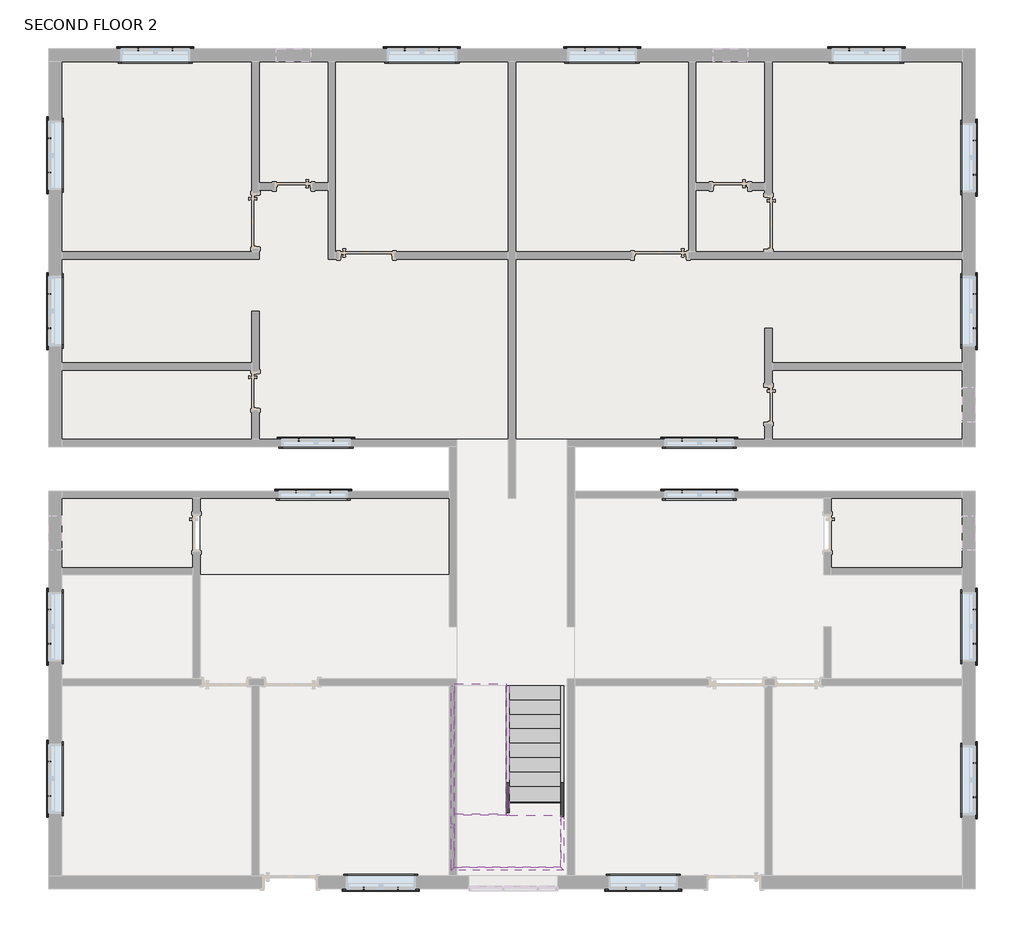
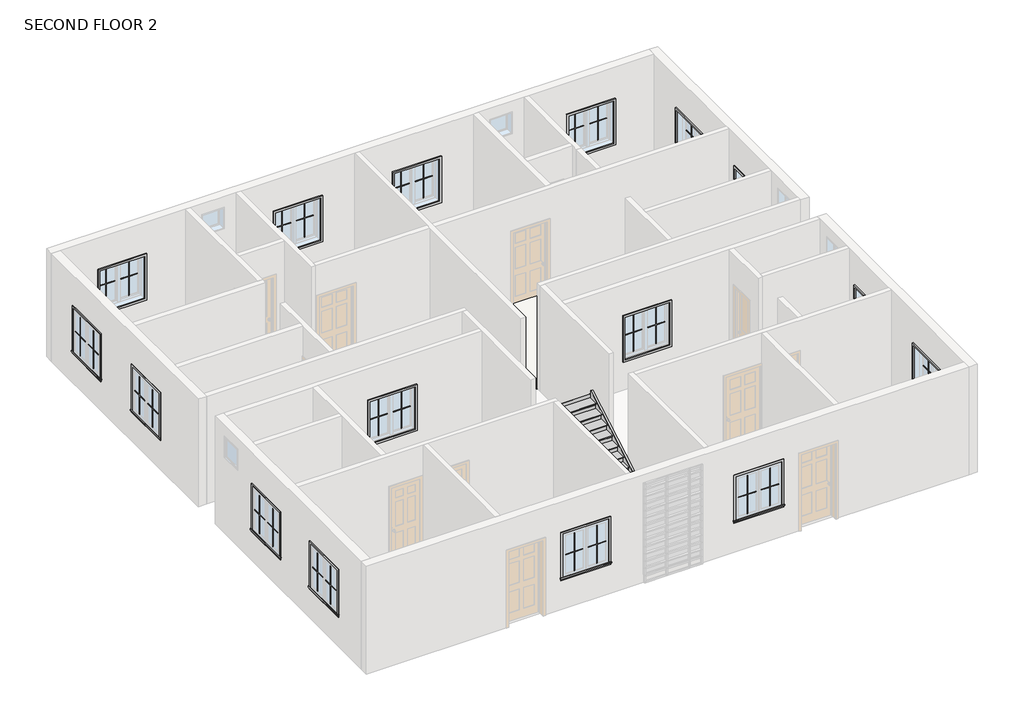
# One storey, part 4 of 4: 72 proxies, 7 members, 4 slabs, 2 stair flights.
"""IFC4 building model written with IfcOpenShell, lengths in millimetres."""

from ifc_helpers import new_model, si_unit, frame, origin, place, context, project, spatial, polyline, outline, extrude, faceted_brep, transform, mapped, element, save
from components import muntin_pattern_2x2_muntin_pattern_2x2_4dfeb3f3, muntin_pattern_2x2_muntin_pattern_2x2_e852a7e4, trim_window_exterior_flat_with_sill_7cfdd449, trim_window_interior_flat_picture_frame_f1e0b15b, non_monolithic_landing_b50a567b, stair_flight_05c21e37, stair_flight_ef5934bc

model = new_model("IFC4")

# Units and contexts
model_context = context("Model", 3, world=origin())
ifc_project = project(units=[si_unit("LENGTHUNIT", "METRE", prefix="MILLI")], contexts=[model_context])

# Site, building, storey
site = spatial("IfcSite", under=ifc_project)
building = spatial("IfcBuilding", under=site)
storey = spatial("IfcBuildingStorey", under=building, Name="SECOND FLOOR 2", Elevation=6343.9725604)

# Proxies
placement = place(None, origin())
muntin_pattern_2x2_muntin_pattern_2x2_shape = muntin_pattern_2x2_muntin_pattern_2x2_4dfeb3f3(model_context)
element("IfcBuildingElementProxy", 1, Name="Muntin Pattern_2x2 : Muntin Pattern_2x2", ObjectType="Muntin Pattern_2x2 : Muntin Pattern_2x2", at=placement, inside=storey, context=model_context, shape_type="MappedRepresentation", body=[
    mapped(muntin_pattern_2x2_muntin_pattern_2x2_shape, transform((-12420.8887331, 2059.7281164, 7328.2225604), x_axis=(0.0, 1.0, 0.0), y_axis=(-1.0, 0.0, 0.0), z_axis=(0.0, 0.0, 1.0))),
])
element("IfcBuildingElementProxy", 2, Name="Muntin Pattern_2x2 : Muntin Pattern_2x2", ObjectType="Muntin Pattern_2x2 : Muntin Pattern_2x2", at=placement, inside=storey, context=model_context, shape_type="MappedRepresentation", body=[
    mapped(muntin_pattern_2x2_muntin_pattern_2x2_shape, transform((-12420.8887331, 4803.7218664, 7328.2225604), x_axis=(0.0, 1.0, 0.0), y_axis=(-1.0, 0.0, 0.0), z_axis=(0.0, 0.0, 1.0))),
])
element("IfcBuildingElementProxy", 3, Name="Muntin Pattern_2x2 : Muntin Pattern_2x2", ObjectType="Muntin Pattern_2x2 : Muntin Pattern_2x2", at=placement, inside=storey, context=model_context, shape_type="MappedRepresentation", body=[
    mapped(muntin_pattern_2x2_muntin_pattern_2x2_shape, transform((-10854.0262331, 6977.8031164, 7328.2225604), x_axis=(1.0, 0.0, 0.0), y_axis=(0.0, 1.0, 0.0), z_axis=(0.0, 0.0, 1.0))),
])
element("IfcBuildingElementProxy", 4, Name="Muntin Pattern_2x2 : Muntin Pattern_2x2", ObjectType="Muntin Pattern_2x2 : Muntin Pattern_2x2", at=placement, inside=storey, context=model_context, shape_type="MappedRepresentation", body=[
    mapped(muntin_pattern_2x2_muntin_pattern_2x2_shape, transform((-6155.0262331, 6977.8031164, 7328.2225604), x_axis=(1.0, 0.0, 0.0), y_axis=(0.0, 1.0, 0.0), z_axis=(0.0, 0.0, 1.0))),
])
element("IfcBuildingElementProxy", 5, Name="Muntin Pattern_2x2 : Muntin Pattern_2x2", ObjectType="Muntin Pattern_2x2 : Muntin Pattern_2x2", at=placement, inside=storey, context=model_context, shape_type="MappedRepresentation", body=[
    mapped(muntin_pattern_2x2_muntin_pattern_2x2_shape, transform((-2980.0262331, 6977.8031164, 7328.2225604), x_axis=(1.0, 0.0, 0.0), y_axis=(0.0, 1.0, 0.0), z_axis=(0.0, 0.0, 1.0))),
])
element("IfcBuildingElementProxy", 6, Name="Muntin Pattern_2x2 : Muntin Pattern_2x2", ObjectType="Muntin Pattern_2x2 : Muntin Pattern_2x2", at=placement, inside=storey, context=model_context, shape_type="MappedRepresentation", body=[
    mapped(muntin_pattern_2x2_muntin_pattern_2x2_shape, transform((1680.8737669, 6977.8031164, 7328.2225604), x_axis=(1.0, 0.0, 0.0), y_axis=(0.0, 1.0, 0.0), z_axis=(0.0, 0.0, 1.0))),
])
element("IfcBuildingElementProxy", 7, Name="Muntin Pattern_2x2 : Muntin Pattern_2x2", ObjectType="Muntin Pattern_2x2 : Muntin Pattern_2x2", at=placement, inside=storey, context=model_context, shape_type="MappedRepresentation", body=[
    mapped(muntin_pattern_2x2_muntin_pattern_2x2_shape, transform((3892.2612669, 5371.2531164, 7328.2225604), x_axis=(0.0, -1.0, 0.0), y_axis=(1.0, 0.0, 0.0), z_axis=(0.0, 0.0, 1.0))),
])
element("IfcBuildingElementProxy", 8, Name="Muntin Pattern_2x2 : Muntin Pattern_2x2", ObjectType="Muntin Pattern_2x2 : Muntin Pattern_2x2", at=placement, inside=storey, context=model_context, shape_type="MappedRepresentation", body=[
    mapped(muntin_pattern_2x2_muntin_pattern_2x2_shape, transform((3892.2612669, 2666.1531164, 7328.2225604), x_axis=(0.0, -1.0, 0.0), y_axis=(1.0, 0.0, 0.0), z_axis=(0.0, 0.0, 1.0))),
])
element("IfcBuildingElementProxy", 9, Name="Muntin Pattern_2x2 : Muntin Pattern_2x2", ObjectType="Muntin Pattern_2x2 : Muntin Pattern_2x2", at=placement, inside=storey, context=model_context, shape_type="MappedRepresentation", body=[
    mapped(muntin_pattern_2x2_muntin_pattern_2x2_shape, transform((3892.2612669, -2896.4468836, 7328.2225604), x_axis=(0.0, -1.0, 0.0), y_axis=(1.0, 0.0, 0.0), z_axis=(0.0, 0.0, 1.0))),
])
element("IfcBuildingElementProxy", 10, Name="Muntin Pattern_2x2 : Muntin Pattern_2x2", ObjectType="Muntin Pattern_2x2 : Muntin Pattern_2x2", at=placement, inside=storey, context=model_context, shape_type="MappedRepresentation", body=[
    mapped(muntin_pattern_2x2_muntin_pattern_2x2_shape, transform((3892.2612669, -5601.5468836, 7328.2225604), x_axis=(0.0, -1.0, 0.0), y_axis=(1.0, 0.0, 0.0), z_axis=(0.0, 0.0, 1.0))),
])
element("IfcBuildingElementProxy", 11, Name="Muntin Pattern_2x2 : Muntin Pattern_2x2", ObjectType="Muntin Pattern_2x2 : Muntin Pattern_2x2", at=placement, inside=storey, context=model_context, shape_type="MappedRepresentation", body=[
    mapped(muntin_pattern_2x2_muntin_pattern_2x2_shape, transform((-1649.7012331, -7812.9343836, 7328.2225604), x_axis=(-1.0, 0.0, 0.0), y_axis=(0.0, -1.0, 0.0), z_axis=(0.0, 0.0, 1.0))),
])
element("IfcBuildingElementProxy", 12, Name="Muntin Pattern_2x2 : Muntin Pattern_2x2", ObjectType="Muntin Pattern_2x2 : Muntin Pattern_2x2", at=placement, inside=storey, context=model_context, shape_type="MappedRepresentation", body=[
    mapped(muntin_pattern_2x2_muntin_pattern_2x2_shape, transform((-6272.5012331, -7812.9343836, 7328.2225604), x_axis=(-1.0, 0.0, 0.0), y_axis=(0.0, -1.0, 0.0), z_axis=(0.0, 0.0, 1.0))),
])
element("IfcBuildingElementProxy", 13, Name="Muntin Pattern_2x2 : Muntin Pattern_2x2", ObjectType="Muntin Pattern_2x2 : Muntin Pattern_2x2", at=placement, inside=storey, context=model_context, shape_type="MappedRepresentation", body=[
    mapped(muntin_pattern_2x2_muntin_pattern_2x2_shape, transform((-12420.8887331, -6182.5718836, 7328.2225604), x_axis=(0.0, 1.0, 0.0), y_axis=(-1.0, 0.0, 0.0), z_axis=(0.0, 0.0, 1.0))),
])
element("IfcBuildingElementProxy", 14, Name="Muntin Pattern_2x2 : Muntin Pattern_2x2", ObjectType="Muntin Pattern_2x2 : Muntin Pattern_2x2", at=placement, inside=storey, context=model_context, shape_type="MappedRepresentation", body=[
    mapped(muntin_pattern_2x2_muntin_pattern_2x2_shape, transform((-12420.8887331, -3502.8718836, 7328.2225604), x_axis=(0.0, 1.0, 0.0), y_axis=(-1.0, 0.0, 0.0), z_axis=(0.0, 0.0, 1.0))),
])
element("IfcBuildingElementProxy", 15, Name="Muntin Pattern_2x2 : Muntin Pattern_2x2", ObjectType="Muntin Pattern_2x2 : Muntin Pattern_2x2", at=placement, inside=storey, context=model_context, shape_type="MappedRepresentation", body=[
    mapped(muntin_pattern_2x2_muntin_pattern_2x2_shape, transform((-8072.7262331, -821.5843836, 7328.2225604), x_axis=(1.0, 0.0, 0.0), y_axis=(0.0, 1.0, 0.0), z_axis=(0.0, 0.0, 1.0))),
])
element("IfcBuildingElementProxy", 16, Name="Muntin Pattern_2x2 : Muntin Pattern_2x2", ObjectType="Muntin Pattern_2x2 : Muntin Pattern_2x2", at=placement, inside=storey, context=model_context, shape_type="MappedRepresentation", body=[
    mapped(muntin_pattern_2x2_muntin_pattern_2x2_shape, transform((-8021.9262331, 92.8156164, 7328.2225604), x_axis=(1.0, 0.0, 0.0), y_axis=(0.0, 1.0, 0.0), z_axis=(0.0, 0.0, 1.0))),
])
element("IfcBuildingElementProxy", 17, Name="Muntin Pattern_2x2 : Muntin Pattern_2x2", ObjectType="Muntin Pattern_2x2 : Muntin Pattern_2x2", at=placement, inside=storey, context=model_context, shape_type="MappedRepresentation", body=[
    mapped(muntin_pattern_2x2_muntin_pattern_2x2_shape, transform((-1265.5262331, -821.5843836, 7328.2225604), x_axis=(1.0, 0.0, 0.0), y_axis=(0.0, 1.0, 0.0), z_axis=(0.0, 0.0, 1.0))),
])
element("IfcBuildingElementProxy", 18, Name="Muntin Pattern_2x2 : Muntin Pattern_2x2", ObjectType="Muntin Pattern_2x2 : Muntin Pattern_2x2", at=placement, inside=storey, context=model_context, shape_type="MappedRepresentation", body=[
    mapped(muntin_pattern_2x2_muntin_pattern_2x2_shape, transform((-1265.5262331, 92.8156164, 7328.2225604), x_axis=(1.0, 0.0, 0.0), y_axis=(0.0, 1.0, 0.0), z_axis=(0.0, 0.0, 1.0))),
])
muntin_pattern_2x2_muntin_pattern_2x2_2_shape = muntin_pattern_2x2_muntin_pattern_2x2_e852a7e4(model_context)
element("IfcBuildingElementProxy", 19, Name="Muntin Pattern_2x2 : Muntin Pattern_2x2", ObjectType="Muntin Pattern_2x2 : Muntin Pattern_2x2", at=placement, inside=storey, context=model_context, shape_type="MappedRepresentation", body=[
    mapped(muntin_pattern_2x2_muntin_pattern_2x2_2_shape, transform((-12420.8887331, 2666.1531164, 7328.2225604), x_axis=(0.0, -1.0, 0.0), y_axis=(1.0, 0.0, 0.0), z_axis=(0.0, 0.0, 1.0))),
])
element("IfcBuildingElementProxy", 20, Name="Muntin Pattern_2x2 : Muntin Pattern_2x2", ObjectType="Muntin Pattern_2x2 : Muntin Pattern_2x2", at=placement, inside=storey, context=model_context, shape_type="MappedRepresentation", body=[
    mapped(muntin_pattern_2x2_muntin_pattern_2x2_2_shape, transform((-12420.8887331, 5410.1468664, 7328.2225604), x_axis=(0.0, -1.0, 0.0), y_axis=(1.0, 0.0, 0.0), z_axis=(0.0, 0.0, 1.0))),
])
element("IfcBuildingElementProxy", 21, Name="Muntin Pattern_2x2 : Muntin Pattern_2x2", ObjectType="Muntin Pattern_2x2 : Muntin Pattern_2x2", at=placement, inside=storey, context=model_context, shape_type="MappedRepresentation", body=[
    mapped(muntin_pattern_2x2_muntin_pattern_2x2_2_shape, transform((-10247.6012331, 6977.8031164, 7328.2225604), x_axis=(-1.0, 0.0, 0.0), y_axis=(0.0, -1.0, 0.0), z_axis=(0.0, 0.0, 1.0))),
])
element("IfcBuildingElementProxy", 22, Name="Muntin Pattern_2x2 : Muntin Pattern_2x2", ObjectType="Muntin Pattern_2x2 : Muntin Pattern_2x2", at=placement, inside=storey, context=model_context, shape_type="MappedRepresentation", body=[
    mapped(muntin_pattern_2x2_muntin_pattern_2x2_2_shape, transform((-5548.6012331, 6977.8031164, 7328.2225604), x_axis=(-1.0, 0.0, 0.0), y_axis=(0.0, -1.0, 0.0), z_axis=(0.0, 0.0, 1.0))),
])
element("IfcBuildingElementProxy", 23, Name="Muntin Pattern_2x2 : Muntin Pattern_2x2", ObjectType="Muntin Pattern_2x2 : Muntin Pattern_2x2", at=placement, inside=storey, context=model_context, shape_type="MappedRepresentation", body=[
    mapped(muntin_pattern_2x2_muntin_pattern_2x2_2_shape, transform((-2373.6012331, 6977.8031164, 7328.2225604), x_axis=(-1.0, 0.0, 0.0), y_axis=(0.0, -1.0, 0.0), z_axis=(0.0, 0.0, 1.0))),
])
element("IfcBuildingElementProxy", 24, Name="Muntin Pattern_2x2 : Muntin Pattern_2x2", ObjectType="Muntin Pattern_2x2 : Muntin Pattern_2x2", at=placement, inside=storey, context=model_context, shape_type="MappedRepresentation", body=[
    mapped(muntin_pattern_2x2_muntin_pattern_2x2_2_shape, transform((2287.2987669, 6977.8031164, 7328.2225604), x_axis=(-1.0, 0.0, 0.0), y_axis=(0.0, -1.0, 0.0), z_axis=(0.0, 0.0, 1.0))),
])
element("IfcBuildingElementProxy", 25, Name="Muntin Pattern_2x2 : Muntin Pattern_2x2", ObjectType="Muntin Pattern_2x2 : Muntin Pattern_2x2", at=placement, inside=storey, context=model_context, shape_type="MappedRepresentation", body=[
    mapped(muntin_pattern_2x2_muntin_pattern_2x2_2_shape, transform((3892.2612669, 4764.8281164, 7328.2225604), x_axis=(0.0, 1.0, 0.0), y_axis=(-1.0, 0.0, 0.0), z_axis=(0.0, 0.0, 1.0))),
])
element("IfcBuildingElementProxy", 26, Name="Muntin Pattern_2x2 : Muntin Pattern_2x2", ObjectType="Muntin Pattern_2x2 : Muntin Pattern_2x2", at=placement, inside=storey, context=model_context, shape_type="MappedRepresentation", body=[
    mapped(muntin_pattern_2x2_muntin_pattern_2x2_2_shape, transform((3892.2612669, 2059.7281164, 7328.2225604), x_axis=(0.0, 1.0, 0.0), y_axis=(-1.0, 0.0, 0.0), z_axis=(0.0, 0.0, 1.0))),
])
element("IfcBuildingElementProxy", 27, Name="Muntin Pattern_2x2 : Muntin Pattern_2x2", ObjectType="Muntin Pattern_2x2 : Muntin Pattern_2x2", at=placement, inside=storey, context=model_context, shape_type="MappedRepresentation", body=[
    mapped(muntin_pattern_2x2_muntin_pattern_2x2_2_shape, transform((3892.2612669, -3502.8718836, 7328.2225604), x_axis=(0.0, 1.0, 0.0), y_axis=(-1.0, 0.0, 0.0), z_axis=(0.0, 0.0, 1.0))),
])
element("IfcBuildingElementProxy", 28, Name="Muntin Pattern_2x2 : Muntin Pattern_2x2", ObjectType="Muntin Pattern_2x2 : Muntin Pattern_2x2", at=placement, inside=storey, context=model_context, shape_type="MappedRepresentation", body=[
    mapped(muntin_pattern_2x2_muntin_pattern_2x2_2_shape, transform((3892.2612669, -6207.9718836, 7328.2225604), x_axis=(0.0, 1.0, 0.0), y_axis=(-1.0, 0.0, 0.0), z_axis=(0.0, 0.0, 1.0))),
])
element("IfcBuildingElementProxy", 29, Name="Muntin Pattern_2x2 : Muntin Pattern_2x2", ObjectType="Muntin Pattern_2x2 : Muntin Pattern_2x2", at=placement, inside=storey, context=model_context, shape_type="MappedRepresentation", body=[
    mapped(muntin_pattern_2x2_muntin_pattern_2x2_2_shape, transform((-2256.1262331, -7812.9343836, 7328.2225604), x_axis=(1.0, 0.0, 0.0), y_axis=(0.0, 1.0, 0.0), z_axis=(0.0, 0.0, 1.0))),
])
element("IfcBuildingElementProxy", 30, Name="Muntin Pattern_2x2 : Muntin Pattern_2x2", ObjectType="Muntin Pattern_2x2 : Muntin Pattern_2x2", at=placement, inside=storey, context=model_context, shape_type="MappedRepresentation", body=[
    mapped(muntin_pattern_2x2_muntin_pattern_2x2_2_shape, transform((-6878.9262331, -7812.9343836, 7328.2225604), x_axis=(1.0, 0.0, 0.0), y_axis=(0.0, 1.0, 0.0), z_axis=(0.0, 0.0, 1.0))),
])
element("IfcBuildingElementProxy", 31, Name="Muntin Pattern_2x2 : Muntin Pattern_2x2", ObjectType="Muntin Pattern_2x2 : Muntin Pattern_2x2", at=placement, inside=storey, context=model_context, shape_type="MappedRepresentation", body=[
    mapped(muntin_pattern_2x2_muntin_pattern_2x2_2_shape, transform((-12420.8887331, -5576.1468836, 7328.2225604), x_axis=(0.0, -1.0, 0.0), y_axis=(1.0, 0.0, 0.0), z_axis=(0.0, 0.0, 1.0))),
])
element("IfcBuildingElementProxy", 32, Name="Muntin Pattern_2x2 : Muntin Pattern_2x2", ObjectType="Muntin Pattern_2x2 : Muntin Pattern_2x2", at=placement, inside=storey, context=model_context, shape_type="MappedRepresentation", body=[
    mapped(muntin_pattern_2x2_muntin_pattern_2x2_2_shape, transform((-12420.8887331, -2896.4468836, 7328.2225604), x_axis=(0.0, -1.0, 0.0), y_axis=(1.0, 0.0, 0.0), z_axis=(0.0, 0.0, 1.0))),
])
element("IfcBuildingElementProxy", 33, Name="Muntin Pattern_2x2 : Muntin Pattern_2x2", ObjectType="Muntin Pattern_2x2 : Muntin Pattern_2x2", at=placement, inside=storey, context=model_context, shape_type="MappedRepresentation", body=[
    mapped(muntin_pattern_2x2_muntin_pattern_2x2_2_shape, transform((-7466.3012331, -821.5843836, 7328.2225604), x_axis=(-1.0, 0.0, 0.0), y_axis=(0.0, -1.0, 0.0), z_axis=(0.0, 0.0, 1.0))),
])
element("IfcBuildingElementProxy", 34, Name="Muntin Pattern_2x2 : Muntin Pattern_2x2", ObjectType="Muntin Pattern_2x2 : Muntin Pattern_2x2", at=placement, inside=storey, context=model_context, shape_type="MappedRepresentation", body=[
    mapped(muntin_pattern_2x2_muntin_pattern_2x2_2_shape, transform((-7415.5012331, 92.8156164, 7328.2225604), x_axis=(-1.0, 0.0, 0.0), y_axis=(0.0, -1.0, 0.0), z_axis=(0.0, 0.0, 1.0))),
])
element("IfcBuildingElementProxy", 35, Name="Muntin Pattern_2x2 : Muntin Pattern_2x2", ObjectType="Muntin Pattern_2x2 : Muntin Pattern_2x2", at=placement, inside=storey, context=model_context, shape_type="MappedRepresentation", body=[
    mapped(muntin_pattern_2x2_muntin_pattern_2x2_2_shape, transform((-659.1012331, -821.5843836, 7328.2225604), x_axis=(-1.0, 0.0, 0.0), y_axis=(0.0, -1.0, 0.0), z_axis=(0.0, 0.0, 1.0))),
])
element("IfcBuildingElementProxy", 36, Name="Muntin Pattern_2x2 : Muntin Pattern_2x2", ObjectType="Muntin Pattern_2x2 : Muntin Pattern_2x2", at=placement, inside=storey, context=model_context, shape_type="MappedRepresentation", body=[
    mapped(muntin_pattern_2x2_muntin_pattern_2x2_2_shape, transform((-659.1012331, 92.8156164, 7328.2225604), x_axis=(-1.0, 0.0, 0.0), y_axis=(0.0, -1.0, 0.0), z_axis=(0.0, 0.0, 1.0))),
])
trim_window_exterior_flat_with_sill_shape = trim_window_exterior_flat_with_sill_7cfdd449(model_context)
element("IfcBuildingElementProxy", 37, Name="Trim-Window-Exterior-Flat : with Sill", ObjectType="Trim-Window-Exterior-Flat : with Sill", at=placement, inside=storey, context=model_context, shape_type="MappedRepresentation", body=[
    mapped(trim_window_exterior_flat_with_sill_shape, transform((-12430.4137331, 2362.9406164, 8477.5725604), x_axis=(0.0, -1.0, 0.0), y_axis=(0.0, 0.0, 1.0), z_axis=(-1.0, 0.0, 0.0))),
])
element("IfcBuildingElementProxy", 38, Name="Trim-Window-Exterior-Flat : with Sill", ObjectType="Trim-Window-Exterior-Flat : with Sill", at=placement, inside=storey, context=model_context, shape_type="MappedRepresentation", body=[
    mapped(trim_window_exterior_flat_with_sill_shape, transform((-12430.4137331, 5106.9343664, 8477.5725604), x_axis=(0.0, -1.0, 0.0), y_axis=(0.0, 0.0, 1.0), z_axis=(-1.0, 0.0, 0.0))),
])
element("IfcBuildingElementProxy", 39, Name="Trim-Window-Exterior-Flat : with Sill", ObjectType="Trim-Window-Exterior-Flat : with Sill", at=placement, inside=storey, context=model_context, shape_type="MappedRepresentation", body=[
    mapped(trim_window_exterior_flat_with_sill_shape, transform((-10550.8137331, 6987.3281164, 8477.5725604), x_axis=(-1.0, 0.0, 0.0), y_axis=(0.0, 0.0, 1.0), z_axis=(0.0, 1.0, 0.0))),
])
element("IfcBuildingElementProxy", 40, Name="Trim-Window-Exterior-Flat : with Sill", ObjectType="Trim-Window-Exterior-Flat : with Sill", at=placement, inside=storey, context=model_context, shape_type="MappedRepresentation", body=[
    mapped(trim_window_exterior_flat_with_sill_shape, transform((-5851.8137331, 6987.3281164, 8477.5725604), x_axis=(-1.0, 0.0, 0.0), y_axis=(0.0, 0.0, 1.0), z_axis=(0.0, 1.0, 0.0))),
])
element("IfcBuildingElementProxy", 41, Name="Trim-Window-Exterior-Flat : with Sill", ObjectType="Trim-Window-Exterior-Flat : with Sill", at=placement, inside=storey, context=model_context, shape_type="MappedRepresentation", body=[
    mapped(trim_window_exterior_flat_with_sill_shape, transform((-2676.8137331, 6987.3281164, 8477.5725604), x_axis=(-1.0, 0.0, 0.0), y_axis=(0.0, 0.0, 1.0), z_axis=(0.0, 1.0, 0.0))),
])
element("IfcBuildingElementProxy", 42, Name="Trim-Window-Exterior-Flat : with Sill", ObjectType="Trim-Window-Exterior-Flat : with Sill", at=placement, inside=storey, context=model_context, shape_type="MappedRepresentation", body=[
    mapped(trim_window_exterior_flat_with_sill_shape, transform((1984.0862669, 6987.3281164, 8477.5725604), x_axis=(-1.0, 0.0, 0.0), y_axis=(0.0, 0.0, 1.0), z_axis=(0.0, 1.0, 0.0))),
])
element("IfcBuildingElementProxy", 43, Name="Trim-Window-Exterior-Flat : with Sill", ObjectType="Trim-Window-Exterior-Flat : with Sill", at=placement, inside=storey, context=model_context, shape_type="MappedRepresentation", body=[
    mapped(trim_window_exterior_flat_with_sill_shape, transform((3901.7862669, 5068.0406164, 8477.5725604), x_axis=(0.0, 1.0, 0.0), y_axis=(0.0, 0.0, 1.0), z_axis=(1.0, 0.0, 0.0))),
])
element("IfcBuildingElementProxy", 44, Name="Trim-Window-Exterior-Flat : with Sill", ObjectType="Trim-Window-Exterior-Flat : with Sill", at=placement, inside=storey, context=model_context, shape_type="MappedRepresentation", body=[
    mapped(trim_window_exterior_flat_with_sill_shape, transform((3901.7862669, 2362.9406164, 8477.5725604), x_axis=(0.0, 1.0, 0.0), y_axis=(0.0, 0.0, 1.0), z_axis=(1.0, 0.0, 0.0))),
])
element("IfcBuildingElementProxy", 45, Name="Trim-Window-Exterior-Flat : with Sill", ObjectType="Trim-Window-Exterior-Flat : with Sill", at=placement, inside=storey, context=model_context, shape_type="MappedRepresentation", body=[
    mapped(trim_window_exterior_flat_with_sill_shape, transform((3901.7862669, -3199.6593836, 8477.5725604), x_axis=(0.0, 1.0, 0.0), y_axis=(0.0, 0.0, 1.0), z_axis=(1.0, 0.0, 0.0))),
])
element("IfcBuildingElementProxy", 46, Name="Trim-Window-Exterior-Flat : with Sill", ObjectType="Trim-Window-Exterior-Flat : with Sill", at=placement, inside=storey, context=model_context, shape_type="MappedRepresentation", body=[
    mapped(trim_window_exterior_flat_with_sill_shape, transform((3901.7862669, -5904.7593836, 8477.5725604), x_axis=(0.0, 1.0, 0.0), y_axis=(0.0, 0.0, 1.0), z_axis=(1.0, 0.0, 0.0))),
])
element("IfcBuildingElementProxy", 47, Name="Trim-Window-Exterior-Flat : with Sill", ObjectType="Trim-Window-Exterior-Flat : with Sill", at=placement, inside=storey, context=model_context, shape_type="MappedRepresentation", body=[
    mapped(trim_window_exterior_flat_with_sill_shape, transform((-1952.9137331, -7822.4593836, 8477.5725604), x_axis=(1.0, 0.0, 0.0), y_axis=(0.0, 0.0, 1.0), z_axis=(0.0, -1.0, 0.0))),
])
element("IfcBuildingElementProxy", 48, Name="Trim-Window-Exterior-Flat : with Sill", ObjectType="Trim-Window-Exterior-Flat : with Sill", at=placement, inside=storey, context=model_context, shape_type="MappedRepresentation", body=[
    mapped(trim_window_exterior_flat_with_sill_shape, transform((-6575.7137331, -7822.4593836, 8477.5725604), x_axis=(1.0, 0.0, 0.0), y_axis=(0.0, 0.0, 1.0), z_axis=(0.0, -1.0, 0.0))),
])
element("IfcBuildingElementProxy", 49, Name="Trim-Window-Exterior-Flat : with Sill", ObjectType="Trim-Window-Exterior-Flat : with Sill", at=placement, inside=storey, context=model_context, shape_type="MappedRepresentation", body=[
    mapped(trim_window_exterior_flat_with_sill_shape, transform((-12430.4137331, -5879.3593836, 8477.5725604), x_axis=(0.0, -1.0, 0.0), y_axis=(0.0, 0.0, 1.0), z_axis=(-1.0, 0.0, 0.0))),
])
element("IfcBuildingElementProxy", 50, Name="Trim-Window-Exterior-Flat : with Sill", ObjectType="Trim-Window-Exterior-Flat : with Sill", at=placement, inside=storey, context=model_context, shape_type="MappedRepresentation", body=[
    mapped(trim_window_exterior_flat_with_sill_shape, transform((-12430.4137331, -3199.6593836, 8477.5725604), x_axis=(0.0, -1.0, 0.0), y_axis=(0.0, 0.0, 1.0), z_axis=(-1.0, 0.0, 0.0))),
])
element("IfcBuildingElementProxy", 51, Name="Trim-Window-Exterior-Flat : with Sill", ObjectType="Trim-Window-Exterior-Flat : with Sill", at=placement, inside=storey, context=model_context, shape_type="MappedRepresentation", body=[
    mapped(trim_window_exterior_flat_with_sill_shape, transform((-7769.5137331, -812.0593836, 8477.5725604), x_axis=(-1.0, 0.0, 0.0), y_axis=(0.0, 0.0, 1.0), z_axis=(0.0, 1.0, 0.0))),
])
element("IfcBuildingElementProxy", 52, Name="Trim-Window-Exterior-Flat : with Sill", ObjectType="Trim-Window-Exterior-Flat : with Sill", at=placement, inside=storey, context=model_context, shape_type="MappedRepresentation", body=[
    mapped(trim_window_exterior_flat_with_sill_shape, transform((-7718.7137331, 102.3406164, 8477.5725604), x_axis=(-1.0, 0.0, 0.0), y_axis=(0.0, 0.0, 1.0), z_axis=(0.0, 1.0, 0.0))),
])
element("IfcBuildingElementProxy", 53, Name="Trim-Window-Exterior-Flat : with Sill", ObjectType="Trim-Window-Exterior-Flat : with Sill", at=placement, inside=storey, context=model_context, shape_type="MappedRepresentation", body=[
    mapped(trim_window_exterior_flat_with_sill_shape, transform((-962.3137331, -812.0593836, 8477.5725604), x_axis=(-1.0, 0.0, 0.0), y_axis=(0.0, 0.0, 1.0), z_axis=(0.0, 1.0, 0.0))),
])
element("IfcBuildingElementProxy", 54, Name="Trim-Window-Exterior-Flat : with Sill", ObjectType="Trim-Window-Exterior-Flat : with Sill", at=placement, inside=storey, context=model_context, shape_type="MappedRepresentation", body=[
    mapped(trim_window_exterior_flat_with_sill_shape, transform((-962.3137331, 102.3406164, 8477.5725604), x_axis=(-1.0, 0.0, 0.0), y_axis=(0.0, 0.0, 1.0), z_axis=(0.0, 1.0, 0.0))),
])
trim_window_interior_flat_picture_frame_shape = trim_window_interior_flat_picture_frame_f1e0b15b(model_context)
element("IfcBuildingElementProxy", 55, Name="Trim-Window-Interior-Flat : Picture Frame", ObjectType="Trim-Window-Interior-Flat : Picture Frame", at=placement, inside=storey, context=model_context, shape_type="MappedRepresentation", body=[
    mapped(trim_window_interior_flat_picture_frame_shape, transform((-12201.8137331, 2362.9406164, 8477.5725604), x_axis=(0.0, 1.0, 0.0), y_axis=(0.0, 0.0, 1.0), z_axis=(1.0, 0.0, 0.0))),
])
element("IfcBuildingElementProxy", 56, Name="Trim-Window-Interior-Flat : Picture Frame", ObjectType="Trim-Window-Interior-Flat : Picture Frame", at=placement, inside=storey, context=model_context, shape_type="MappedRepresentation", body=[
    mapped(trim_window_interior_flat_picture_frame_shape, transform((-12201.8137331, 5106.9343664, 8477.5725604), x_axis=(0.0, 1.0, 0.0), y_axis=(0.0, 0.0, 1.0), z_axis=(1.0, 0.0, 0.0))),
])
element("IfcBuildingElementProxy", 57, Name="Trim-Window-Interior-Flat : Picture Frame", ObjectType="Trim-Window-Interior-Flat : Picture Frame", at=placement, inside=storey, context=model_context, shape_type="MappedRepresentation", body=[
    mapped(trim_window_interior_flat_picture_frame_shape, transform((-10550.8137331, 6758.7281164, 8477.5725604), x_axis=(1.0, 0.0, 0.0), y_axis=(0.0, 0.0, 1.0), z_axis=(0.0, -1.0, 0.0))),
])
element("IfcBuildingElementProxy", 58, Name="Trim-Window-Interior-Flat : Picture Frame", ObjectType="Trim-Window-Interior-Flat : Picture Frame", at=placement, inside=storey, context=model_context, shape_type="MappedRepresentation", body=[
    mapped(trim_window_interior_flat_picture_frame_shape, transform((-5851.8137331, 6758.7281164, 8477.5725604), x_axis=(1.0, 0.0, 0.0), y_axis=(0.0, 0.0, 1.0), z_axis=(0.0, -1.0, 0.0))),
])
element("IfcBuildingElementProxy", 59, Name="Trim-Window-Interior-Flat : Picture Frame", ObjectType="Trim-Window-Interior-Flat : Picture Frame", at=placement, inside=storey, context=model_context, shape_type="MappedRepresentation", body=[
    mapped(trim_window_interior_flat_picture_frame_shape, transform((-2676.8137331, 6758.7281164, 8477.5725604), x_axis=(1.0, 0.0, 0.0), y_axis=(0.0, 0.0, 1.0), z_axis=(0.0, -1.0, 0.0))),
])
element("IfcBuildingElementProxy", 60, Name="Trim-Window-Interior-Flat : Picture Frame", ObjectType="Trim-Window-Interior-Flat : Picture Frame", at=placement, inside=storey, context=model_context, shape_type="MappedRepresentation", body=[
    mapped(trim_window_interior_flat_picture_frame_shape, transform((1984.0862669, 6758.7281164, 8477.5725604), x_axis=(1.0, 0.0, 0.0), y_axis=(0.0, 0.0, 1.0), z_axis=(0.0, -1.0, 0.0))),
])
element("IfcBuildingElementProxy", 61, Name="Trim-Window-Interior-Flat : Picture Frame", ObjectType="Trim-Window-Interior-Flat : Picture Frame", at=placement, inside=storey, context=model_context, shape_type="MappedRepresentation", body=[
    mapped(trim_window_interior_flat_picture_frame_shape, transform((3673.1862669, 5068.0406164, 8477.5725604), x_axis=(0.0, -1.0, 0.0), y_axis=(0.0, 0.0, 1.0), z_axis=(-1.0, 0.0, 0.0))),
])
element("IfcBuildingElementProxy", 62, Name="Trim-Window-Interior-Flat : Picture Frame", ObjectType="Trim-Window-Interior-Flat : Picture Frame", at=placement, inside=storey, context=model_context, shape_type="MappedRepresentation", body=[
    mapped(trim_window_interior_flat_picture_frame_shape, transform((3673.1862669, 2362.9406164, 8477.5725604), x_axis=(0.0, -1.0, 0.0), y_axis=(0.0, 0.0, 1.0), z_axis=(-1.0, 0.0, 0.0))),
])
element("IfcBuildingElementProxy", 63, Name="Trim-Window-Interior-Flat : Picture Frame", ObjectType="Trim-Window-Interior-Flat : Picture Frame", at=placement, inside=storey, context=model_context, shape_type="MappedRepresentation", body=[
    mapped(trim_window_interior_flat_picture_frame_shape, transform((3673.1862669, -3199.6593836, 8477.5725604), x_axis=(0.0, -1.0, 0.0), y_axis=(0.0, 0.0, 1.0), z_axis=(-1.0, 0.0, 0.0))),
])
element("IfcBuildingElementProxy", 64, Name="Trim-Window-Interior-Flat : Picture Frame", ObjectType="Trim-Window-Interior-Flat : Picture Frame", at=placement, inside=storey, context=model_context, shape_type="MappedRepresentation", body=[
    mapped(trim_window_interior_flat_picture_frame_shape, transform((3673.1862669, -5904.7593836, 8477.5725604), x_axis=(0.0, -1.0, 0.0), y_axis=(0.0, 0.0, 1.0), z_axis=(-1.0, 0.0, 0.0))),
])
element("IfcBuildingElementProxy", 65, Name="Trim-Window-Interior-Flat : Picture Frame", ObjectType="Trim-Window-Interior-Flat : Picture Frame", at=placement, inside=storey, context=model_context, shape_type="MappedRepresentation", body=[
    mapped(trim_window_interior_flat_picture_frame_shape, transform((-1952.9137331, -7593.8593836, 8477.5725604), x_axis=(-1.0, 0.0, 0.0), y_axis=(0.0, 0.0, 1.0), z_axis=(0.0, 1.0, 0.0))),
])
element("IfcBuildingElementProxy", 66, Name="Trim-Window-Interior-Flat : Picture Frame", ObjectType="Trim-Window-Interior-Flat : Picture Frame", at=placement, inside=storey, context=model_context, shape_type="MappedRepresentation", body=[
    mapped(trim_window_interior_flat_picture_frame_shape, transform((-6575.7137331, -7593.8593836, 8477.5725604), x_axis=(-1.0, 0.0, 0.0), y_axis=(0.0, 0.0, 1.0), z_axis=(0.0, 1.0, 0.0))),
])
element("IfcBuildingElementProxy", 67, Name="Trim-Window-Interior-Flat : Picture Frame", ObjectType="Trim-Window-Interior-Flat : Picture Frame", at=placement, inside=storey, context=model_context, shape_type="MappedRepresentation", body=[
    mapped(trim_window_interior_flat_picture_frame_shape, transform((-12201.8137331, -5879.3593836, 8477.5725604), x_axis=(0.0, 1.0, 0.0), y_axis=(0.0, 0.0, 1.0), z_axis=(1.0, 0.0, 0.0))),
])
element("IfcBuildingElementProxy", 68, Name="Trim-Window-Interior-Flat : Picture Frame", ObjectType="Trim-Window-Interior-Flat : Picture Frame", at=placement, inside=storey, context=model_context, shape_type="MappedRepresentation", body=[
    mapped(trim_window_interior_flat_picture_frame_shape, transform((-12201.8137331, -3199.6593836, 8477.5725604), x_axis=(0.0, 1.0, 0.0), y_axis=(0.0, 0.0, 1.0), z_axis=(1.0, 0.0, 0.0))),
])
element("IfcBuildingElementProxy", 69, Name="Trim-Window-Interior-Flat : Picture Frame", ObjectType="Trim-Window-Interior-Flat : Picture Frame", at=placement, inside=storey, context=model_context, shape_type="MappedRepresentation", body=[
    mapped(trim_window_interior_flat_picture_frame_shape, transform((-7769.5137331, -939.0593836, 8477.5725604), x_axis=(1.0, 0.0, 0.0), y_axis=(0.0, 0.0, 1.0), z_axis=(0.0, -1.0, 0.0))),
])
element("IfcBuildingElementProxy", 70, Name="Trim-Window-Interior-Flat : Picture Frame", ObjectType="Trim-Window-Interior-Flat : Picture Frame", at=placement, inside=storey, context=model_context, shape_type="MappedRepresentation", body=[
    mapped(trim_window_interior_flat_picture_frame_shape, transform((-7718.7137331, -24.6593836, 8477.5725604), x_axis=(1.0, 0.0, 0.0), y_axis=(0.0, 0.0, 1.0), z_axis=(0.0, -1.0, 0.0))),
])
element("IfcBuildingElementProxy", 71, Name="Trim-Window-Interior-Flat : Picture Frame", ObjectType="Trim-Window-Interior-Flat : Picture Frame", at=placement, inside=storey, context=model_context, shape_type="MappedRepresentation", body=[
    mapped(trim_window_interior_flat_picture_frame_shape, transform((-962.3137331, -939.0593836, 8477.5725604), x_axis=(1.0, 0.0, 0.0), y_axis=(0.0, 0.0, 1.0), z_axis=(0.0, -1.0, 0.0))),
])
element("IfcBuildingElementProxy", 72, Name="Trim-Window-Interior-Flat : Picture Frame", ObjectType="Trim-Window-Interior-Flat : Picture Frame", at=placement, inside=storey, context=model_context, shape_type="MappedRepresentation", body=[
    mapped(trim_window_interior_flat_picture_frame_shape, transform((-962.3137331, -24.6593836, 8477.5725604), x_axis=(1.0, 0.0, 0.0), y_axis=(0.0, 0.0, 1.0), z_axis=(0.0, -1.0, 0.0))),
])

# Members
element("IfcMember", 73, ObjectType="Stringer - 2\" Width", at=placement, inside=storey, context=model_context, shape_type="SweptSolid", body=[
    extrude(outline(polyline([(-4241.0593836, 6553.8933656), (-4241.0593836, 6343.9725604), (-4486.3086974, 6343.9725604), (-6633.5807846, 7593.8618174), (-6551.3310691, 7898.6618174), (-4241.0593836, 6553.8933656)])), frame((-3400.7137331, 0.0, 0.0), z_axis=(1.0, 0.0, 0.0), x_axis=(0.0, 1.0, 0.0)), (0.0, 0.0, 1.0), 50.8),
])
element("IfcMember", 74, ObjectType="Stringer - 2\" Width", at=placement, inside=storey, context=model_context, shape_type="SweptSolid", body=[
    extrude(outline(polyline([(-4241.0593836, 6553.8933656), (-4241.0593836, 6343.9725604), (-4486.3086974, 6343.9725604), (-6476.2593836, 7502.2878011), (-6476.2593836, 7854.9639117), (-4241.0593836, 6553.8933656)])), frame((-4365.9137331, 0.0, 0.0), z_axis=(1.0, 0.0, 0.0), x_axis=(0.0, 1.0, 0.0)), (0.0, 0.0, 1.0), 50.8),
])
element("IfcMember", 75, ObjectType="Stringer - 2\" Width", at=placement, inside=storey, context=model_context, shape_type="SweptSolid", body=[
    extrude(outline(polyline([(-6674.5379826, 7593.8618174), (-6756.7876981, 7898.6618174), (-4241.0593836, 9363.0229538), (-4241.0593836, 9010.3468432), (-6674.5379826, 7593.8618174)])), frame((-5331.1137331, 0.0, 0.0), z_axis=(1.0, 0.0, 0.0), x_axis=(0.0, 1.0, 0.0)), (0.0, 0.0, 1.0), 50.8),
])
element("IfcMember", 76, ObjectType="Stringer - 2\" Width", at=placement, inside=storey, context=model_context, shape_type="SweptSolid", body=[
    extrude(outline(polyline([(-6527.0593836, 7679.706512), (-6527.0593836, 8032.3826225), (-4241.0593836, 9363.0229538), (-4241.0593836, 9010.3468432), (-6527.0593836, 7679.706512)])), frame((-4365.9137331, 0.0, 0.0), z_axis=(1.0, 0.0, 0.0), x_axis=(0.0, 1.0, 0.0)), (0.0, 0.0, 1.0), 50.8),
])
element("IfcMember", 77, ObjectType="Stringer - 2\" Width", at=placement, inside=storey, context=model_context, shape_type="Brep", body=[
    faceted_brep([(-5280.3137331, -6756.7876981, 7898.6618174), (-5331.1137331, -6756.7876981, 7898.6618174), (-5331.1137331, -7492.2593836, 7898.6618174), (-5280.3137331, -7441.4593836, 7898.6618174), (-5280.3137331, -6674.5379826, 7593.8618174), (-5280.3137331, -7441.4593836, 7593.8618174), (-5331.1137331, -6674.5379826, 7593.8618174), (-5331.1137331, -7492.2593836, 7593.8618174)], [[[0, 1, 2, 3]], [[4, 0, 3, 5]], [[6, 4, 5, 7]], [[1, 6, 7, 2]], [[1, 0, 4, 6]], [[2, 7, 5, 3]]]),
])
element("IfcMember", 78, ObjectType="Stringer - 2\" Width", at=placement, inside=storey, context=model_context, shape_type="SweptSolid", body=[
    extrude(outline(polyline([(-5331.1137331, -7492.2593836), (-5280.3137331, -7441.4593836), (-3400.7137331, -7441.4593836), (-3349.9137331, -7492.2593836), (-5331.1137331, -7492.2593836)])), frame((0.0, 0.0, 7593.8618174), z_axis=(0.0, 0.0, 1.0), x_axis=(1.0, 0.0, 0.0)), (0.0, 0.0, 1.0), 304.8),
])
element("IfcMember", 79, ObjectType="Stringer - 2\" Width", at=placement, inside=storey, context=model_context, shape_type="Brep", body=[
    faceted_brep([(-3400.7137331, -7441.4593836, 7898.6618174), (-3349.9137331, -7492.2593836, 7898.6618174), (-3349.9137331, -6551.3310691, 7898.6618174), (-3400.7137331, -6551.3310691, 7898.6618174), (-3400.7137331, -7441.4593836, 7593.8618174), (-3400.7137331, -6633.5807846, 7593.8618174), (-3349.9137331, -7492.2593836, 7593.8618174), (-3349.9137331, -6633.5807846, 7593.8618174)], [[[0, 1, 2, 3]], [[4, 0, 3, 5]], [[6, 4, 5, 7]], [[1, 6, 7, 2]], [[1, 0, 4, 6]], [[2, 7, 5, 3]]]),
])

# Slabs
non_monolithic_landing_shape = non_monolithic_landing_b50a567b(model_context)
element("IfcSlab", 80, ObjectType="Non-Monolithic Landing", at=placement, inside=storey, context=model_context, shape_type="MappedRepresentation", body=[
    mapped(non_monolithic_landing_shape, transform((0.0, 0.0, 0.0), x_axis=(1.0, 0.0, 0.0), y_axis=(0.0, 1.0, 0.0), z_axis=(0.0, 0.0, 1.0))),
])
element("IfcSlab", 81, ObjectType="marble tiles", at=placement, inside=storey, context=model_context, shape_type="SweptSolid", body=[
    extrude(outline(polyline([(-9890.4137331, -939.0593836), (-9890.4137331, -2158.2593836), (-12201.8137331, -2158.2593836), (-12201.8137331, -939.0593836), (-9890.4137331, -939.0593836)])), frame((0.0, 0.0, 6248.4), z_axis=(0.0, 0.0, 1.0), x_axis=(1.0, 0.0, 0.0)), (0.0, 0.0, 1.0), 152.4),
    extrude(outline(polyline([(3673.1862669, -2158.2593836), (1361.7862669, -2158.2593836), (1361.7862669, -939.0593836), (3673.1862669, -939.0593836), (3673.1862669, -2158.2593836)])), frame((0.0, 0.0, 6248.4), z_axis=(0.0, 0.0, 1.0), x_axis=(1.0, 0.0, 0.0)), (0.0, 0.0, 1.0), 152.4),
    extrude(outline(polyline([(-7502.8137331, 6758.7281164), (-7502.8137331, 4623.5406164), (-8722.0137331, 4623.5406164), (-8722.0137331, 6758.7281164), (-7502.8137331, 6758.7281164)])), frame((0.0, 0.0, 6248.4), z_axis=(0.0, 0.0, 1.0), x_axis=(1.0, 0.0, 0.0)), (0.0, 0.0, 1.0), 152.4),
    extrude(outline(polyline([(193.3862669, 4623.5406164), (-1025.8137331, 4623.5406164), (-1025.8137331, 6758.7281164), (193.3862669, 6758.7281164), (193.3862669, 4623.5406164)])), frame((0.0, 0.0, 6248.4), z_axis=(0.0, 0.0, 1.0), x_axis=(1.0, 0.0, 0.0)), (0.0, 0.0, 1.0), 152.4),
])
element("IfcSlab", 82, ObjectType="marble tiles", at=placement, inside=storey, context=model_context, shape_type="SweptSolid", body=[
    extrude(outline(polyline([(3673.1862669, 102.3406164), (-12201.8137331, 102.3406164), (-12201.8137331, 6758.7281164), (3673.1862669, 6758.7281164), (3673.1862669, 102.3406164)])), frame((0.0, 0.0, 6248.4), z_axis=(0.0, 0.0, 1.0), x_axis=(1.0, 0.0, 0.0)), (0.0, 0.0, 1.0), 152.4),
])
element("IfcSlab", 83, ObjectType="marble tiles", at=placement, inside=storey, context=model_context, shape_type="SweptSolid", body=[
    extrude(outline(polyline([(-5242.2137331, -2285.2593836), (-9763.4137331, -2285.2593836), (-9763.4137331, -812.0593836), (-5242.2137331, -812.0593836), (-5242.2137331, -2285.2593836)])), frame((0.0, 0.0, 6248.4), z_axis=(0.0, 0.0, 1.0), x_axis=(1.0, 0.0, 0.0)), (0.0, 0.0, 1.0), 152.4),
])

# Stair flights
stair_flight_shape = stair_flight_05c21e37(model_context)
element("IfcStairFlight", 84, ObjectType="2\" Tread 1\" Nosing 1/4\" Riser", at=placement, inside=storey, context=model_context, shape_type="MappedRepresentation", body=[
    mapped(stair_flight_shape, transform((0.0, 0.0, 0.0), x_axis=(1.0, 0.0, 0.0), y_axis=(0.0, 1.0, 0.0), z_axis=(0.0, 0.0, 1.0))),
])
stair_flight_2_shape = stair_flight_ef5934bc(model_context)
element("IfcStairFlight", 85, ObjectType="2\" Tread 1\" Nosing 1/4\" Riser", at=placement, inside=storey, context=model_context, shape_type="MappedRepresentation", body=[
    mapped(stair_flight_2_shape, transform((0.0, 0.0, 0.0), x_axis=(1.0, 0.0, 0.0), y_axis=(0.0, 1.0, 0.0), z_axis=(0.0, 0.0, 1.0))),
])

save(model, "model.ifc")

# Revit data of these elements
# Type "Muntin Pattern_2x2 : Muntin Pattern_2x2"
#   Width [instance default] = 4' - 0"
#   Thickness = 0' - 0 1/2"
#   Height [instance default] = 4' - 0"
#   Distance = 0' - 0 3/4"
#   Interior Material [instance default] = none
#   Exterior Material [instance default] = none
#   Default Elevation = 0
# Type "Trim-Window-Exterior-Flat : with Sill"
#   Trim Width = 0' - 2 1/4"
#   Trim Thickness_Picture Frame = 0' - 1 1/4"
#   Trim Thickness_with Sill = 0' - 0 3/4"
#   Sill Thickness = 0' - 1 1/4"
#   Opening Width [instance default] = 2' - 0"
#   Opening Height [instance default] = 3' - 0"
#   Default Elevation = 4' - 0"
#   Sill = yes
#   Picture Frame = no
#   Trim Material [instance default] = none
# Type "Trim-Window-Interior-Flat : Picture Frame"
#   Trim Thickness_Picture Frame = 0' - 1 1/4"
#   Trim Width = 0' - 2 1/4"
#   Trim Thickness_with Sill = 0' - 0 3/4"
#   Sill Thickness = 0' - 1 1/4"
#   Opening Width [instance default] = 2' - 0"
#   Opening Height [instance default] = 3' - 0"
#   Default Elevation = 4' - 0"
#   Sill = no
#   Picture Frame = yes
#   Trim Material [instance default] = none
# Type "marble tiles"
#   Assembly Code = "B1010"
#   Function = 0
#   Layers, outside or top first: 0' - 6" "marble flooring" (function 1)
# Elements 1, 2, 3, 4, 5, 6, 7, 8, 9, 10, 11, 12, 13, 14, 15, 16, 17, 18, 19, 20, 21, 22, 23, 24, 25, 26, 27, 28, 29, 30, 31, 32, 33, 34, 35, 36 (IfcBuildingElementProxy, "Muntin Pattern_2x2 : Muntin Pattern_2x2")
#   Width = 1' - 6 5/8"
#   Height = 3' - 6 1/2"
#   Interior Material = Wood - Stained
#   Exterior Material = Clad - White
#   Phase Created = New Construction
#   Materials on its faces: "Clad - White", "Wood - Stained"
# Elements 37, 38, 39, 40, 41, 42, 43, 44, 45, 46, 47, 48, 49, 50, 51, 52, 53, 54 (IfcBuildingElementProxy, "Trim-Window-Exterior-Flat : with Sill")
#   Opening Width = 4' - 0"
#   Opening Height = 4' - 0"
#   Trim Material = Clad - White
#   Phase Created = New Construction
#   Materials on its faces: "Clad - White"
# Elements 55, 56, 57, 58, 59, 60, 61, 62, 63, 64, 65, 66, 67, 68, 69, 70, 71, 72 (IfcBuildingElementProxy, "Trim-Window-Interior-Flat : Picture Frame")
#   Opening Width = 4' - 0"
#   Opening Height = 4' - 0"
#   Trim Material = Wood - Stained
#   Phase Created = New Construction
#   Materials on its faces: "Wood - Stained"
# Elements 73, 74, 75, 76, 77, 78, 79 (IfcMember, "Stringer - 2\" Width")
#   Phase Created = New Construction
# Element 80 (IfcSlab, "Non-Monolithic Landing")
#   Phase Created = New Construction
# Elements 81, 82, 83 (IfcSlab, "marble tiles")
#   Height Offset From Level = 0' - 2.2373"
#   Phase Created = New Construction
#   Materials on its faces: "marble flooring"
# Elements 84, 85 (IfcStairFlight, "2\" Tread 1\" Nosing 1/4\" Riser")
#   Phase Created = New Construction
# Materials
#   "marble flooring": class "Generic", colour RGB 120 120 120, transparency 0, Cost = 0
#   "Clad - White": class "Wood", colour RGB 242 242 238, transparency 0, Cost = 0
#   "Wood - Stained": class "Wood", colour RGB 224 178 126, transparency 0, Cost = 0
